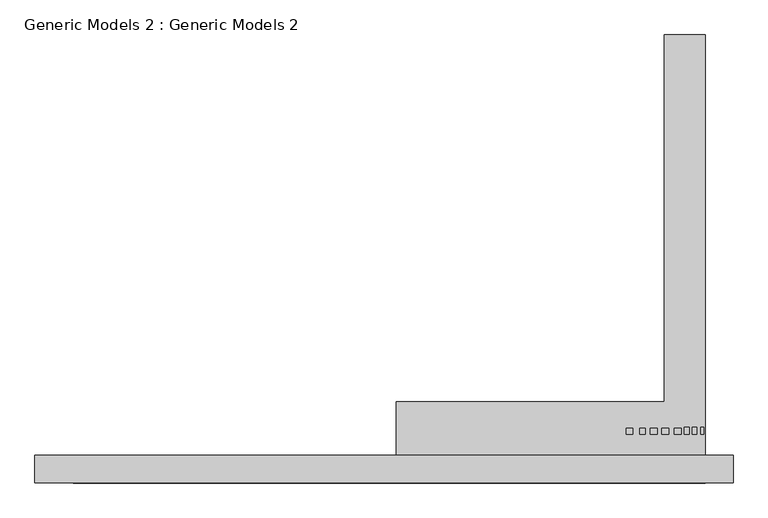
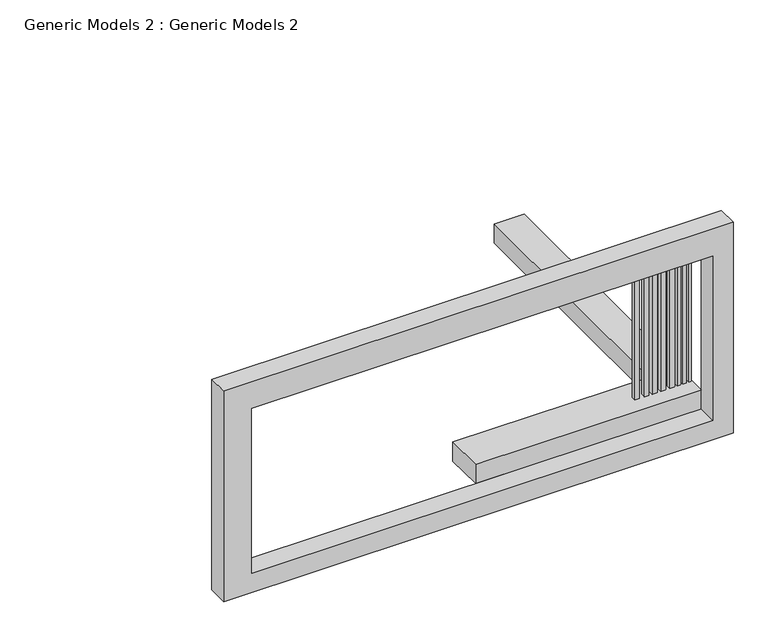
"""IFC4 building model written with IfcOpenShell, lengths in millimetres: proxy geometry, Generic Models 2 : Generic Models 2."""

from ifc_helpers import new_model, si_unit, frame, origin, place, context, project, spatial, polyline, outline, extrude, source, transform, mapped, element, save


def generic_models_2_generic_models_2_9ece3dfc(model_context):
    return source(origin(), model_context, "Body", "SweptSolid", [
        extrude(outline(polyline([(-8925.8628107, -13816.2642965), (-12316.7628107, -13816.2642965), (-12316.7628107, -13228.9081727), (-9375.5621833, -13228.9081727), (-9375.5621833, -9206.1642965), (-8925.8628107, -9206.1642965), (-8925.8628107, -13816.2642965)])), frame((0.0, 0.0, 3352.8), z_axis=(0.0, 0.0, 1.0), x_axis=(1.0, 0.0, 0.0)), (0.0, 0.0, 1.0), 304.8),
        extrude(outline(polyline([(-9103.6628107, -13587.6642965), (-9154.4628107, -13587.6642965), (-9154.4628107, -13511.4642965), (-9103.6628107, -13511.4642965), (-9103.6628107, -13587.6642965)])), frame((0.0, 0.0, 3657.6), z_axis=(0.0, 0.0, 1.0), x_axis=(1.0, 0.0, 0.0)), (0.0, 0.0, 1.0), 2438.4),
        extrude(outline(polyline([(-9017.2311735, -13587.6642965), (-9069.6107692, -13587.6642965), (-9069.6107692, -13511.4642965), (-9017.2311735, -13511.4642965), (-9017.2311735, -13587.6642965)])), frame((0.0, 0.0, 3657.6), z_axis=(0.0, 0.0, 1.0), x_axis=(1.0, 0.0, 0.0)), (0.0, 0.0, 1.0), 2438.4),
        extrude(outline(polyline([(-8943.4909114, -13511.4642965), (-8943.4909114, -13587.6642965), (-8977.4949284, -13587.6642965), (-8977.4949284, -13511.4642965), (-8943.4909114, -13511.4642965)])), frame((0.0, 0.0, 3657.6), z_axis=(0.0, 0.0, 1.0), x_axis=(1.0, 0.0, 0.0)), (0.0, 0.0, 1.0), 2438.4),
        extrude(outline(polyline([(-9532.0361009, -13587.6642965), (-9532.0361009, -13518.1585678), (-9455.1639541, -13518.1585678), (-9455.1639541, -13587.6642965), (-9532.0361009, -13587.6642965)])), frame((0.0, 0.0, 3657.6), z_axis=(0.0, 0.0, 1.0), x_axis=(1.0, 0.0, 0.0)), (0.0, 0.0, 1.0), 2438.4),
        extrude(outline(polyline([(-9646.0909709, -13587.6642965), (-9646.0909709, -13518.1585678), (-9582.9101155, -13518.1585678), (-9582.9101155, -13587.6642965), (-9646.0909709, -13587.6642965)])), frame((0.0, 0.0, 3657.6), z_axis=(0.0, 0.0, 1.0), x_axis=(1.0, 0.0, 0.0)), (0.0, 0.0, 1.0), 2438.4),
        extrude(outline(polyline([(-9791.4069383, -13587.6642965), (-9791.4069383, -13518.1585678), (-9721.9079974, -13518.1585678), (-9721.9079974, -13587.6642965), (-9791.4069383, -13587.6642965)])), frame((0.0, 0.0, 3657.6), z_axis=(0.0, 0.0, 1.0), x_axis=(1.0, 0.0, 0.0)), (0.0, 0.0, 1.0), 2438.4),
        extrude(outline(polyline([(-9327.1829159, -13518.1585678), (-9327.1829159, -13587.6642965), (-9401.2323116, -13587.6642965), (-9401.2323116, -13518.1585678), (-9327.1829159, -13518.1585678)])), frame((0.0, 0.0, 3657.6), z_axis=(0.0, 0.0, 1.0), x_axis=(1.0, 0.0, 0.0)), (0.0, 0.0, 1.0), 2438.4),
        extrude(outline(polyline([(-9191.0275753, -13587.6642965), (-9265.0769711, -13587.6642965), (-9265.0769711, -13518.1585678), (-9191.0275753, -13518.1585678), (-9191.0275753, -13587.6642965)])), frame((0.0, 0.0, 3657.6), z_axis=(0.0, 0.0, 1.0), x_axis=(1.0, 0.0, 0.0)), (0.0, 0.0, 1.0), 2438.4),
        extrude(outline(polyline([(3048.0, -8621.0628107), (6400.8, -8621.0628107), (6400.8, -16279.1628107), (3048.0, -16279.1628107), (3048.0, -8621.0628107)]), holes=[polyline([(3352.8, -15860.0628107), (5970.1200183, -15860.0628107), (5970.1200183, -8925.8628107), (3352.8, -8925.8628107), (3352.8, -15860.0628107)])]), frame((0.0, -14121.0642965, 0.0), z_axis=(0.0, 1.0, 0.0), x_axis=(0.0, 0.0, 1.0)), (0.0, 0.0, 1.0), 304.8),
    ])


if __name__ == "__main__":
    model = new_model("IFC4")
    model_context = context("Model", 3, world=origin())
    ifc_project = project(units=[si_unit("LENGTHUNIT", "METRE", prefix="MILLI")], contexts=[model_context])
    site = spatial("IfcSite", under=ifc_project)
    building = spatial("IfcBuilding", under=site)
    placement = place(None, origin())
    generic_models_2_generic_models_2_shape = generic_models_2_generic_models_2_9ece3dfc(model_context)
    element("IfcBuildingElementProxy", 1, Name="Generic Models 2 : Generic Models 2", ObjectType="Generic Models 2 : Generic Models 2", at=placement, inside=building, context=model_context, shape_type="MappedRepresentation", body=[
        mapped(generic_models_2_generic_models_2_shape, transform((0.0, 0.0, 0.0), x_axis=(1.0, 0.0, 0.0), y_axis=(0.0, 1.0, 0.0), z_axis=(0.0, 0.0, 1.0))),
    ])
    save(model, "model.ifc")
